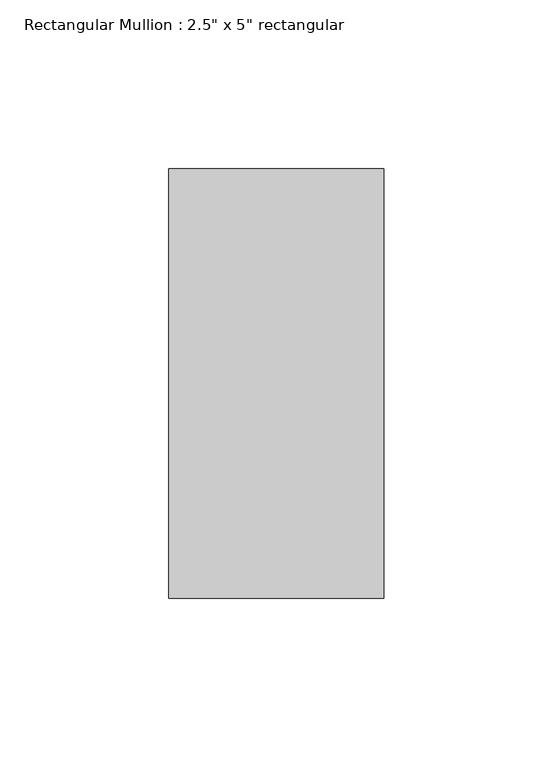
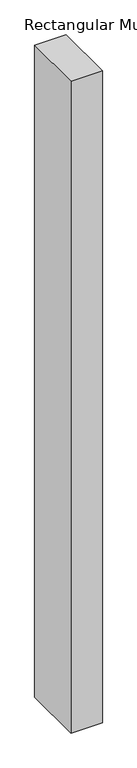
"""IFC4 building model written with IfcOpenShell, lengths in millimetres: member geometry."""

from ifc_helpers import new_model, si_unit, frame, origin, place, context, project, spatial, polyline, outline, extrude, source, transform, mapped, element, save


def member_950090be(model_context):
    return source(origin(), model_context, "Body", "SweptSolid", [
        extrude(outline(polyline([(31.75, 63.5), (31.75, -63.5), (-31.75, -63.5), (-31.75, 63.5), (31.75, 63.5)])), frame((0.0, 0.0, -1394.8833333), z_axis=(0.0, 0.0, 1.0), x_axis=(1.0, 0.0, 0.0)), (0.0, 0.0, 1.0), 1394.8833333),
    ])


if __name__ == "__main__":
    model = new_model("IFC4")
    model_context = context("Model", 3, world=origin())
    ifc_project = project(units=[si_unit("LENGTHUNIT", "METRE", prefix="MILLI")], contexts=[model_context])
    site = spatial("IfcSite", under=ifc_project)
    building = spatial("IfcBuilding", under=site)
    placement = place(None, origin())
    member_shape = member_950090be(model_context)
    element("IfcMember", 1, ObjectType="Rectangular Mullion : 2.5\" x 5\" rectangular", at=placement, inside=building, context=model_context, shape_type="MappedRepresentation", body=[
        mapped(member_shape, transform((0.0, 0.0, 0.0), x_axis=(1.0, 0.0, 0.0), y_axis=(0.0, 1.0, 0.0), z_axis=(0.0, 0.0, 1.0))),
    ])
    save(model, "model.ifc")

# Revit data of these elements
# Type "Rectangular Mullion : 2.5\" x 5\" rectangular"
#   built-in parameter 1007304 = 0.416667 (stored number, unit not read)
#   built-in parameter 1007301 = 0.104167 (stored number, unit not read)
#   built-in parameter 1007300 = 0.104167 (stored number, unit not read)
# Element 1 (IfcMember, "Rectangular Mullion : 2.5\" x 5\" rectangular")
#   Materials on its faces: "Aluminum"
# Materials
#   "Aluminum": class "Metal", colour RGB 247 247 247, transparency 0, Description = "Aluminum 6061", Cost = 0
